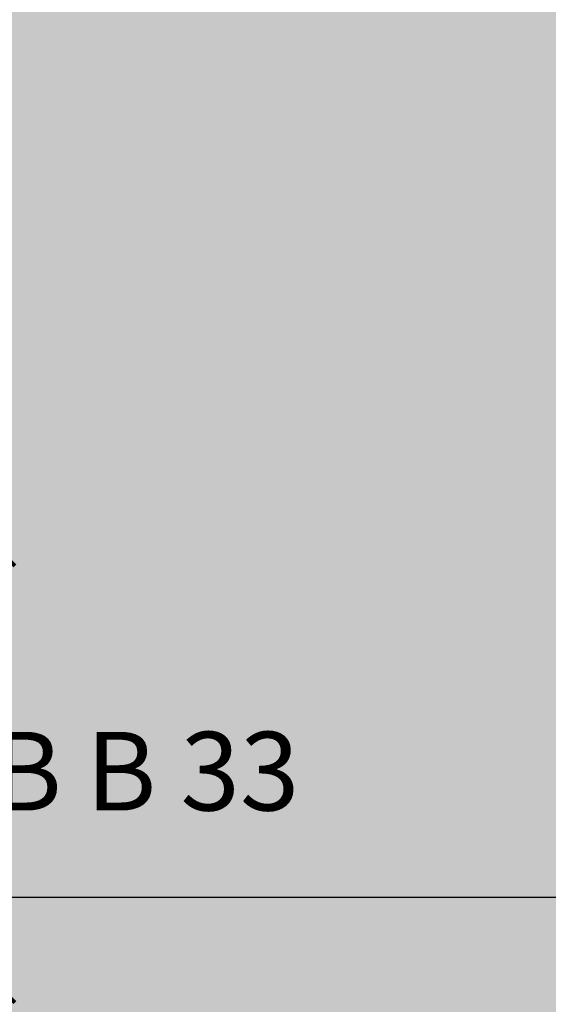
# Model space of a CAD drawing. Units: inches. Extents: x 1704 to 6393, y -157 to 1172.
# Tile 14 of 122: x 1934 to 1975, y 82 to 157. Entities that reach past the tile are written whole.
import ezdxf

# ---------------------------------------------------------------- set-up
doc = ezdxf.new("R2010")
doc.units = ezdxf.units.IN
doc.header["$MEASUREMENT"] = 0
doc.layers.add('A-ANNO-DIMS', color=7, linetype='Continuous', lineweight=13)
doc.layers.add('L-PLNT-PATT', color=253, linetype='Continuous', lineweight=13, true_color=0x9abc8f)
doc.styles.get("Standard").update_dxf_attribs({"font": 'arial.ttf'})
doc.dimstyles.get("Standard").update_dxf_attribs({"dimtxt": 6, "dimasz": 2, "dimexe": 0.18, "dimexo": 0.0625, "dimgap": 0.09, "dimtad": 0, "dimtih": 1, "dimtoh": 1, "dimdec": 1, "dimzin": 0, "dimdsep": 46, "dimlunit": 3, "dimtxsty": 'Standard', "dimblk": 'ARCHTICK', "dimcen": 0.09, "dimadec": 0, "dimazin": 0, "dimtfac": 1, "dimtdec": 1, "dimtofl": 0, "dimtmove": 0, "dimatfit": 3, "dimfxl": 1, "dimtolj": 1, "dimtzin": 0, "dimarcsym": 0})

# ---------------------------------------------------------------- blocks, each defined once
blk = doc.blocks.new('_ArchTick')
at = {"color": 0, "linetype": 'ByBlock', "const_width": 0.15}
blk.add_lwpolyline([(-0.5, -0.5), (0.5, 0.5)], dxfattribs=at)
blk = doc.blocks.new('*D82')
at = {"layer": 'A-ANNO-DIMS', "color": 0, "lineweight": -2, "transparency": 16777216}
for p, q in [((1927.934, 116.512), (1933.05, 116.512)), ((1932.87, 116.512), (1932.87, 103.044)), ((1932.87, 83.187), (1932.87, 96.655)), ((1927.934, 83.187), (1933.05, 83.187))]:
    blk.add_line(p, q, dxfattribs=at)
at = {"layer": 'Defpoints', "color": 0, "lineweight": -3, "transparency": 16777216}
for p in [(1927.871, 116.512), (1927.871, 83.187), (1932.87, 83.187)]:
    blk.add_point(p, dxfattribs=at)
at = {"layer": 'A-ANNO-DIMS', "color": 0, "lineweight": -2, "transparency": 16777216, "xscale": 2, "yscale": 2, "zscale": 2}
for p, rotation in [((1932.87, 116.512), 90), ((1932.87, 83.187), 270)]:
    blk.add_blockref('_ArchTick', p, dxfattribs=dict(at, rotation=rotation))
at = {"layer": 'A-ANNO-DIMS', "color": 0, "transparency": 16777216, "insert": (1932.87, 99.849), "char_height": 6, "attachment_point": 5}
blk.add_mtext('\\A1;SHRUB B 33', dxfattribs=at)
blk = doc.blocks.new('*D93')
at = {"layer": 'A-ANNO-DIMS', "color": 0, "lineweight": -2, "transparency": 16777216}
for p, q in [((2605.286, 895.213), (1829.698, 895.213)), ((1829.878, 895.213), (1829.878, 495.866)), ((1829.878, 90.213), (1829.878, 489.56)), ((2605.286, 90.213), (1829.698, 90.213))]:
    blk.add_line(p, q, dxfattribs=at)
at = {"layer": 'Defpoints', "color": 0, "lineweight": -3, "transparency": 16777216}
for p in [(2605.349, 895.213), (1829.878, 90.213), (2605.349, 90.213)]:
    blk.add_point(p, dxfattribs=at)
at = {"layer": 'A-ANNO-DIMS', "color": 0, "lineweight": -2, "transparency": 16777216, "xscale": 2, "yscale": 2, "zscale": 2}
for p, rotation in [((1829.878, 895.213), 90), ((1829.878, 90.213), 270)]:
    blk.add_blockref('_ArchTick', p, dxfattribs=dict(at, rotation=rotation))
at = {"layer": 'A-ANNO-DIMS', "color": 0, "transparency": 16777216, "insert": (1829.878, 492.713), "char_height": 6, "attachment_point": 5}
blk.add_mtext('\\A1;805', dxfattribs=at)

msp = doc.modelspace()

# ---------------------------------------------------------------- hatches: boundary and pattern name
at = {"layer": 'L-PLNT-PATT', "transparency": 33554643}
h = msp.add_hatch(color=256, dxfattribs=at)
h.dxf.hatch_style = 1
h.paths.add_polyline_path([(1975.349, 202.213), (1898.349, 202.213), (1898.349, -3.787), (1975.349, -3.787)])

# ---------------------------------------------------------------- dimensions: what is measured, and where the dimension line sits
at = {"layer": 'A-ANNO-DIMS'}
dim = msp.add_linear_dim(base=(1829.878, 90.213), p1=(2605.349, 895.213), p2=(2605.349, 90.213), angle=90, dimstyle='Standard', override={"dimdec": 0, "dimlfac": 1, "dimrnd": 0, "dimzin": 0, "dimdsep": 46, "dimlunit": 2}, dxfattribs=at)
dim.commit()
dim.dimension.update_dxf_attribs({"geometry": '*D93', "text_midpoint": (1829.878, 492.713)})
dim = msp.add_linear_dim(base=(1932.87, 83.187), p1=(1927.871, 116.512), p2=(1927.871, 83.187), angle=270, text='SHRUB B <>', dimstyle='Standard', override={"dimdec": 0, "dimlfac": 1, "dimrnd": 0, "dimzin": 0, "dimdsep": 46, "dimlunit": 2}, dxfattribs=at)
dim.commit()
dim.dimension.update_dxf_attribs({"geometry": '*D82', "text_midpoint": (1932.87, 99.849)})

doc.saveas('drawing.dxf')
